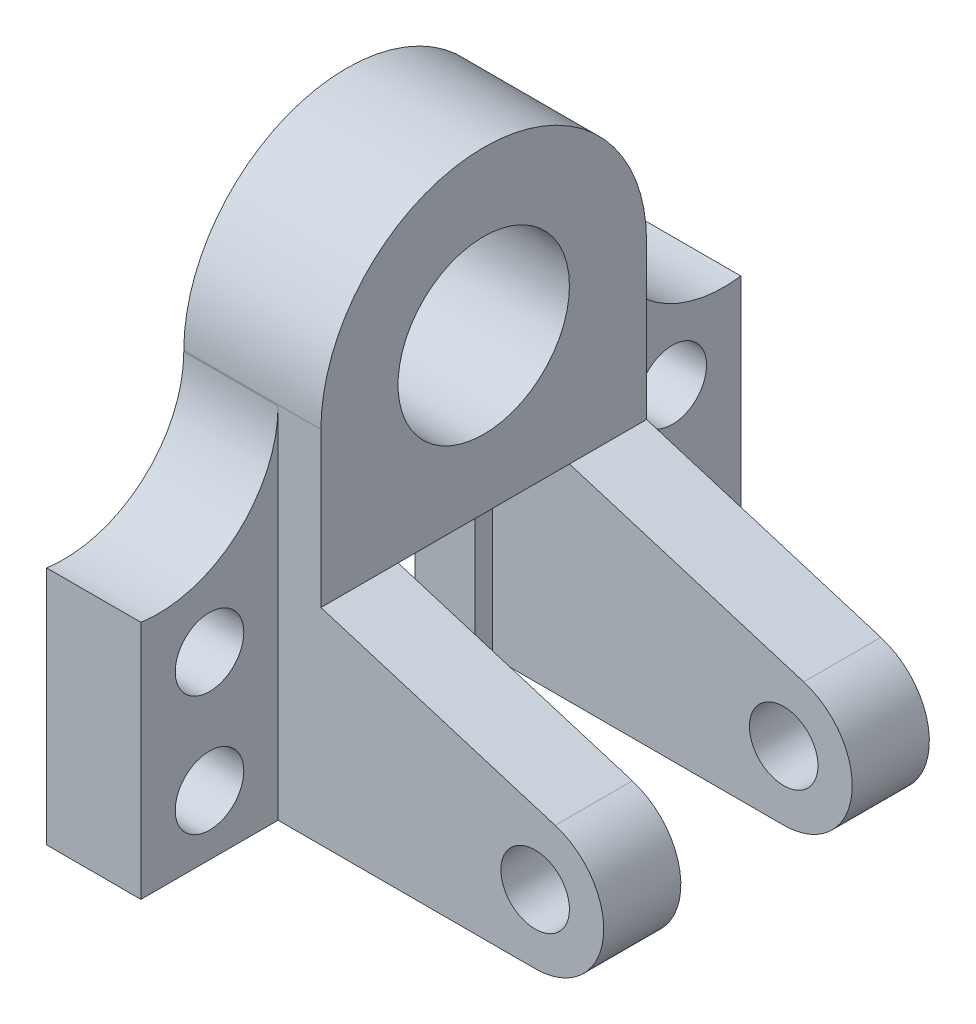
ISO-10303-21;
HEADER;
FILE_DESCRIPTION(('STEP AP214'),'2;1');
FILE_NAME('part.step','',(''),(''),'','','');
FILE_SCHEMA(('AUTOMOTIVE_DESIGN { 1 0 10303 214 1 1 1 1 }'));
ENDSEC;
DATA;
#1=APPLICATION_CONTEXT('core data for automotive mechanical design processes');
#2=APPLICATION_PROTOCOL_DEFINITION('international standard','automotive_design',2000,#1);
#3=PRODUCT_CONTEXT('',#1,'mechanical');
#4=PRODUCT('Part','Part','',(#3));
#5=PRODUCT_RELATED_PRODUCT_CATEGORY('part','',(#4));
#6=PRODUCT_DEFINITION_FORMATION('','',#4);
#7=PRODUCT_DEFINITION_CONTEXT('part definition',#1,'design');
#8=PRODUCT_DEFINITION('design','',#6,#7);
#9=PRODUCT_DEFINITION_SHAPE('','',#8);
#10=(LENGTH_UNIT() NAMED_UNIT(*) SI_UNIT(.MILLI.,.METRE.));
#11=(NAMED_UNIT(*) PLANE_ANGLE_UNIT() SI_UNIT($,.RADIAN.));
#12=(NAMED_UNIT(*) SI_UNIT($,.STERADIAN.) SOLID_ANGLE_UNIT());
#13=UNCERTAINTY_MEASURE_WITH_UNIT(LENGTH_MEASURE(1.E-05),#10,'distance_accuracy_value','');
#14=(GEOMETRIC_REPRESENTATION_CONTEXT(3) GLOBAL_UNCERTAINTY_ASSIGNED_CONTEXT((#13)) GLOBAL_UNIT_ASSIGNED_CONTEXT((#10,
#11,#12)) REPRESENTATION_CONTEXT('',''));
#15=CARTESIAN_POINT('',(0.,0.,0.));
#16=DIRECTION('',(0.,0.,1.));
#17=DIRECTION('',(1.,0.,0.));
#18=AXIS2_PLACEMENT_3D('',#15,#16,#17);
#19=CARTESIAN_POINT('',(32.,-36.,38.));
#20=DIRECTION('',(0.,1.,0.));
#21=DIRECTION('',(0.,0.,1.));
#22=AXIS2_PLACEMENT_3D('',#19,#20,#21);
#23=PLANE('',#22);
#24=DIRECTION('',(0.,0.,-1.));
#25=VECTOR('',#24,1.);
#26=CARTESIAN_POINT('',(14.,-36.,20.));
#27=LINE('',#26,#25);
#28=CARTESIAN_POINT('',(14.,-36.,20.));
#29=VERTEX_POINT('',#28);
#30=CARTESIAN_POINT('',(14.,-36.,16.));
#31=VERTEX_POINT('',#30);
#32=EDGE_CURVE('E181',#29,#31,#27,.T.);
#33=ORIENTED_EDGE('',*,*,#32,.T.);
#34=DIRECTION('',(-1.,0.,0.));
#35=VECTOR('',#34,1.);
#36=CARTESIAN_POINT('',(14.,-36.,16.));
#37=LINE('',#36,#35);
#38=CARTESIAN_POINT('',(0.,-36.,16.));
#39=VERTEX_POINT('',#38);
#40=EDGE_CURVE('E730',#31,#39,#37,.T.);
#41=ORIENTED_EDGE('',*,*,#40,.T.);
#42=DIRECTION('',(0.,0.,-1.));
#43=VECTOR('',#42,1.);
#44=CARTESIAN_POINT('',(0.,-36.,38.));
#45=LINE('',#44,#43);
#46=CARTESIAN_POINT('',(0.,-36.,-16.));
#47=VERTEX_POINT('',#46);
#48=EDGE_CURVE('E61',#39,#47,#45,.T.);
#49=ORIENTED_EDGE('',*,*,#48,.T.);
#50=DIRECTION('',(-1.,0.,0.));
#51=VECTOR('',#50,1.);
#52=CARTESIAN_POINT('',(14.,-36.,-16.));
#53=LINE('',#52,#51);
#54=CARTESIAN_POINT('',(14.,-36.,-16.));
#55=VERTEX_POINT('',#54);
#56=EDGE_CURVE('E57',#55,#47,#53,.T.);
#57=ORIENTED_EDGE('',*,*,#56,.F.);
#58=DIRECTION('',(0.,0.,-1.));
#59=VECTOR('',#58,1.);
#60=CARTESIAN_POINT('',(14.,-36.,-20.));
#61=LINE('',#60,#59);
#62=CARTESIAN_POINT('',(14.,-36.,-20.));
#63=VERTEX_POINT('',#62);
#64=EDGE_CURVE('E744',#55,#63,#61,.T.);
#65=ORIENTED_EDGE('',*,*,#64,.T.);
#66=DIRECTION('',(-1.,0.,0.));
#67=VECTOR('',#66,1.);
#68=CARTESIAN_POINT('',(32.,-36.,-20.));
#69=LINE('',#68,#67);
#70=CARTESIAN_POINT('',(32.,-36.,-20.));
#71=VERTEX_POINT('',#70);
#72=EDGE_CURVE('E368',#71,#63,#69,.T.);
#73=ORIENTED_EDGE('',*,*,#72,.F.);
#74=DIRECTION('',(0.,0.,-1.));
#75=VECTOR('',#74,1.);
#76=CARTESIAN_POINT('',(32.,-36.,38.));
#77=LINE('',#76,#75);
#78=CARTESIAN_POINT('',(32.,-36.,20.));
#79=VERTEX_POINT('',#78);
#80=EDGE_CURVE('E206',#79,#71,#77,.T.);
#81=ORIENTED_EDGE('',*,*,#80,.F.);
#82=DIRECTION('',(-1.,0.,0.));
#83=VECTOR('',#82,1.);
#84=CARTESIAN_POINT('',(32.,-36.,20.));
#85=LINE('',#84,#83);
#86=EDGE_CURVE('E200',#79,#29,#85,.T.);
#87=ORIENTED_EDGE('',*,*,#86,.T.);
#88=EDGE_LOOP('',(#33,#41,#49,#57,#65,#73,#81,#87));
#89=FACE_BOUND('',#88,.T.);
#90=ADVANCED_FACE('F41',(#89),#23,.F.);
#91=CARTESIAN_POINT('',(32.,0.,-38.));
#92=DIRECTION('',(0.,0.,1.));
#93=DIRECTION('',(0.,-1.,0.));
#94=AXIS2_PLACEMENT_3D('',#91,#92,#93);
#95=PLANE('',#94);
#96=DIRECTION('',(0.,-1.,0.));
#97=VECTOR('',#96,1.);
#98=CARTESIAN_POINT('',(22.,-0.28718707889796,-38.));
#99=LINE('',#98,#97);
#100=CARTESIAN_POINT('',(22.,-0.28718707889796,-38.));
#101=VERTEX_POINT('',#100);
#102=CARTESIAN_POINT('',(22.,-84.,-38.));
#103=VERTEX_POINT('',#102);
#104=EDGE_CURVE('E238',#101,#103,#99,.T.);
#105=ORIENTED_EDGE('',*,*,#104,.F.);
#106=DIRECTION('',(-1.,0.,0.));
#107=VECTOR('',#106,1.);
#108=CARTESIAN_POINT('',(22.,-0.28718707889796,-38.));
#109=LINE('',#108,#107);
#110=CARTESIAN_POINT('',(0.,-0.287187078897948,-38.));
#111=VERTEX_POINT('',#110);
#112=EDGE_CURVE('E260',#101,#111,#109,.T.);
#113=ORIENTED_EDGE('',*,*,#112,.T.);
#114=DIRECTION('',(0.,1.,0.));
#115=VECTOR('',#114,1.);
#116=CARTESIAN_POINT('',(0.,0.,-38.));
#117=LINE('',#116,#115);
#118=CARTESIAN_POINT('',(0.,0.,-38.));
#119=VERTEX_POINT('',#118);
#120=EDGE_CURVE('E307',#111,#119,#117,.T.);
#121=ORIENTED_EDGE('',*,*,#120,.T.);
#122=DIRECTION('',(-1.,0.,0.));
#123=VECTOR('',#122,1.);
#124=CARTESIAN_POINT('',(32.,0.,-38.));
#125=LINE('',#124,#123);
#126=CARTESIAN_POINT('',(32.,0.,-38.));
#127=VERTEX_POINT('',#126);
#128=EDGE_CURVE('E47',#127,#119,#125,.T.);
#129=ORIENTED_EDGE('',*,*,#128,.F.);
#130=DIRECTION('',(0.,1.,0.));
#131=VECTOR('',#130,1.);
#132=CARTESIAN_POINT('',(32.,0.,-38.));
#133=LINE('',#132,#131);
#134=CARTESIAN_POINT('',(32.,-36.,-38.));
#135=VERTEX_POINT('',#134);
#136=EDGE_CURVE('E313',#135,#127,#133,.T.);
#137=ORIENTED_EDGE('',*,*,#136,.F.);
#138=DIRECTION('',(-0.956390801813646,0.292090113160734,0.));
#139=VECTOR('',#138,1.);
#140=CARTESIAN_POINT('',(86.6734418105717,-52.6977471709817,-38.));
#141=LINE('',#140,#139);
#142=CARTESIAN_POINT('',(86.6734418105717,-52.6977471709817,-38.));
#143=VERTEX_POINT('',#142);
#144=EDGE_CURVE('E348',#143,#135,#141,.T.);
#145=ORIENTED_EDGE('',*,*,#144,.F.);
#146=CARTESIAN_POINT('',(82.,-68.,-38.));
#147=DIRECTION('',(0.,0.,1.));
#148=DIRECTION('',(1.,0.,0.));
#149=AXIS2_PLACEMENT_3D('',#146,#147,#148);
#150=CIRCLE('',#149,16.);
#151=CARTESIAN_POINT('',(82.,-84.,-38.));
#152=VERTEX_POINT('',#151);
#153=EDGE_CURVE('E352',#152,#143,#150,.T.);
#154=ORIENTED_EDGE('',*,*,#153,.F.);
#155=DIRECTION('',(1.,0.,0.));
#156=VECTOR('',#155,1.);
#157=CARTESIAN_POINT('',(0.,-84.,-38.));
#158=LINE('',#157,#156);
#159=EDGE_CURVE('E365',#103,#152,#158,.T.);
#160=ORIENTED_EDGE('',*,*,#159,.F.);
#161=EDGE_LOOP('',(#105,#113,#121,#129,#137,#145,#154,#160));
#162=FACE_BOUND('',#161,.T.);
#163=CARTESIAN_POINT('',(82.,-68.,-38.));
#164=DIRECTION('',(0.,0.,1.));
#165=DIRECTION('',(1.,0.,0.));
#166=AXIS2_PLACEMENT_3D('',#163,#164,#165);
#167=CIRCLE('',#166,8.00000000000001);
#168=CARTESIAN_POINT('',(90.,-68.,-38.));
#169=VERTEX_POINT('',#168);
#170=EDGE_CURVE('E373',#169,#169,#167,.T.);
#171=ORIENTED_EDGE('',*,*,#170,.T.);
#172=EDGE_LOOP('',(#171));
#173=FACE_BOUND('',#172,.T.);
#174=ADVANCED_FACE('F350',(#162,#173),#95,.F.);
#175=CARTESIAN_POINT('',(32.,0.,0.));
#176=DIRECTION('',(1.,0.,0.));
#177=DIRECTION('',(0.,0.,-1.));
#178=AXIS2_PLACEMENT_3D('',#175,#176,#177);
#179=PLANE('',#178);
#180=CARTESIAN_POINT('',(32.,0.,0.));
#181=DIRECTION('',(1.,0.,0.));
#182=DIRECTION('',(0.,0.,-1.));
#183=AXIS2_PLACEMENT_3D('',#180,#181,#182);
#184=CIRCLE('',#183,38.);
#185=CARTESIAN_POINT('',(32.,0.,38.));
#186=VERTEX_POINT('',#185);
#187=EDGE_CURVE('E301',#127,#186,#184,.T.);
#188=ORIENTED_EDGE('',*,*,#187,.T.);
#189=DIRECTION('',(0.,-1.,0.));
#190=VECTOR('',#189,1.);
#191=CARTESIAN_POINT('',(32.,0.,38.));
#192=LINE('',#191,#190);
#193=CARTESIAN_POINT('',(32.,-36.,38.));
#194=VERTEX_POINT('',#193);
#195=EDGE_CURVE('E308',#186,#194,#192,.T.);
#196=ORIENTED_EDGE('',*,*,#195,.T.);
#197=EDGE_CURVE('E310',#194,#79,#77,.T.);
#198=ORIENTED_EDGE('',*,*,#197,.T.);
#199=ORIENTED_EDGE('',*,*,#80,.T.);
#200=DIRECTION('',(0.,0.,1.));
#201=VECTOR('',#200,1.);
#202=CARTESIAN_POINT('',(32.,-36.,-38.));
#203=LINE('',#202,#201);
#204=EDGE_CURVE('E342',#135,#71,#203,.T.);
#205=ORIENTED_EDGE('',*,*,#204,.F.);
#206=ORIENTED_EDGE('',*,*,#136,.T.);
#207=EDGE_LOOP('',(#188,#196,#198,#199,#205,#206));
#208=FACE_BOUND('',#207,.T.);
#209=CARTESIAN_POINT('',(32.,0.,0.));
#210=DIRECTION('',(1.,0.,0.));
#211=DIRECTION('',(0.,0.,-1.));
#212=AXIS2_PLACEMENT_3D('',#209,#210,#211);
#213=CIRCLE('',#212,20.);
#214=CARTESIAN_POINT('',(32.,0.,-20.));
#215=VERTEX_POINT('',#214);
#216=EDGE_CURVE('E300',#215,#215,#213,.T.);
#217=ORIENTED_EDGE('',*,*,#216,.F.);
#218=EDGE_LOOP('',(#217));
#219=FACE_BOUND('',#218,.T.);
#220=ADVANCED_FACE('F343',(#208,#219),#179,.T.);
#221=CARTESIAN_POINT('',(0.,0.,0.));
#222=DIRECTION('',(1.,0.,0.));
#223=DIRECTION('',(0.,0.,-1.));
#224=AXIS2_PLACEMENT_3D('',#221,#222,#223);
#225=PLANE('',#224);
#226=ORIENTED_EDGE('',*,*,#48,.F.);
#227=DIRECTION('',(0.,-1.,0.));
#228=VECTOR('',#227,1.);
#229=CARTESIAN_POINT('',(0.,-36.,16.));
#230=LINE('',#229,#228);
#231=CARTESIAN_POINT('',(0.,-84.,16.));
#232=VERTEX_POINT('',#231);
#233=EDGE_CURVE('E205',#39,#232,#230,.T.);
#234=ORIENTED_EDGE('',*,*,#233,.T.);
#235=DIRECTION('',(0.,0.,-1.));
#236=VECTOR('',#235,1.);
#237=CARTESIAN_POINT('',(0.,-84.,38.));
#238=LINE('',#237,#236);
#239=CARTESIAN_POINT('',(0.,-84.,70.));
#240=VERTEX_POINT('',#239);
#241=EDGE_CURVE('E280',#240,#232,#238,.T.);
#242=ORIENTED_EDGE('',*,*,#241,.F.);
#243=DIRECTION('',(0.,-1.,0.));
#244=VECTOR('',#243,1.);
#245=CARTESIAN_POINT('',(0.,-28.,70.));
#246=LINE('',#245,#244);
#247=CARTESIAN_POINT('',(0.,-28.,70.));
#248=VERTEX_POINT('',#247);
#249=EDGE_CURVE('E288',#248,#240,#246,.T.);
#250=ORIENTED_EDGE('',*,*,#249,.F.);
#251=CARTESIAN_POINT('',(0.,-0.287187078897969,66.));
#252=DIRECTION('',(-1.,0.,0.));
#253=DIRECTION('',(0.,0.,-1.));
#254=AXIS2_PLACEMENT_3D('',#251,#252,#253);
#255=CIRCLE('',#254,28.);
#256=CARTESIAN_POINT('',(0.,-0.287187078897969,38.));
#257=VERTEX_POINT('',#256);
#258=EDGE_CURVE('E269',#257,#248,#255,.T.);
#259=ORIENTED_EDGE('',*,*,#258,.F.);
#260=DIRECTION('',(0.,-1.,0.));
#261=VECTOR('',#260,1.);
#262=CARTESIAN_POINT('',(0.,0.,38.));
#263=LINE('',#262,#261);
#264=CARTESIAN_POINT('',(0.,0.,38.));
#265=VERTEX_POINT('',#264);
#266=EDGE_CURVE('E312',#265,#257,#263,.T.);
#267=ORIENTED_EDGE('',*,*,#266,.F.);
#268=CARTESIAN_POINT('',(0.,0.,0.));
#269=DIRECTION('',(1.,0.,0.));
#270=DIRECTION('',(0.,0.,-1.));
#271=AXIS2_PLACEMENT_3D('',#268,#269,#270);
#272=CIRCLE('',#271,38.);
#273=EDGE_CURVE('E299',#119,#265,#272,.T.);
#274=ORIENTED_EDGE('',*,*,#273,.F.);
#275=ORIENTED_EDGE('',*,*,#120,.F.);
#276=CARTESIAN_POINT('',(0.,-0.287187078897953,-66.));
#277=DIRECTION('',(-1.,0.,0.));
#278=DIRECTION('',(0.,0.,1.));
#279=AXIS2_PLACEMENT_3D('',#276,#277,#278);
#280=CIRCLE('',#279,28.);
#281=CARTESIAN_POINT('',(0.,-28.,-70.));
#282=VERTEX_POINT('',#281);
#283=EDGE_CURVE('E234',#282,#111,#280,.T.);
#284=ORIENTED_EDGE('',*,*,#283,.F.);
#285=DIRECTION('',(0.,1.,0.));
#286=VECTOR('',#285,1.);
#287=CARTESIAN_POINT('',(0.,-28.,-70.));
#288=LINE('',#287,#286);
#289=CARTESIAN_POINT('',(0.,-84.,-70.));
#290=VERTEX_POINT('',#289);
#291=EDGE_CURVE('E241',#290,#282,#288,.T.);
#292=ORIENTED_EDGE('',*,*,#291,.F.);
#293=DIRECTION('',(0.,0.,-1.));
#294=VECTOR('',#293,1.);
#295=CARTESIAN_POINT('',(0.,-84.,-38.));
#296=LINE('',#295,#294);
#297=CARTESIAN_POINT('',(0.,-84.,-16.));
#298=VERTEX_POINT('',#297);
#299=EDGE_CURVE('E247',#298,#290,#296,.T.);
#300=ORIENTED_EDGE('',*,*,#299,.F.);
#301=DIRECTION('',(0.,1.,0.));
#302=VECTOR('',#301,1.);
#303=CARTESIAN_POINT('',(0.,-84.,-16.));
#304=LINE('',#303,#302);
#305=EDGE_CURVE('E733',#298,#47,#304,.T.);
#306=ORIENTED_EDGE('',*,*,#305,.T.);
#307=EDGE_LOOP('',(#226,#234,#242,#250,#259,#267,#274,#275,#284,#292,#300,#306));
#308=FACE_BOUND('',#307,.T.);
#309=CARTESIAN_POINT('',(0.,0.,0.));
#310=DIRECTION('',(1.,0.,0.));
#311=DIRECTION('',(0.,0.,-1.));
#312=AXIS2_PLACEMENT_3D('',#309,#310,#311);
#313=CIRCLE('',#312,20.);
#314=CARTESIAN_POINT('',(0.,0.,-20.));
#315=VERTEX_POINT('',#314);
#316=EDGE_CURVE('E296',#315,#315,#313,.T.);
#317=ORIENTED_EDGE('',*,*,#316,.T.);
#318=EDGE_LOOP('',(#317));
#319=FACE_BOUND('',#318,.T.);
#320=CARTESIAN_POINT('',(0.,-42.,54.));
#321=DIRECTION('',(1.,0.,0.));
#322=DIRECTION('',(0.,0.,-1.));
#323=AXIS2_PLACEMENT_3D('',#320,#321,#322);
#324=CIRCLE('',#323,8.);
#325=CARTESIAN_POINT('',(0.,-42.,46.));
#326=VERTEX_POINT('',#325);
#327=EDGE_CURVE('E262',#326,#326,#324,.T.);
#328=ORIENTED_EDGE('',*,*,#327,.T.);
#329=EDGE_LOOP('',(#328));
#330=FACE_BOUND('',#329,.T.);
#331=CARTESIAN_POINT('',(0.,-70.,54.));
#332=DIRECTION('',(1.,0.,0.));
#333=DIRECTION('',(0.,0.,-1.));
#334=AXIS2_PLACEMENT_3D('',#331,#332,#333);
#335=CIRCLE('',#334,8.);
#336=CARTESIAN_POINT('',(0.,-70.,46.));
#337=VERTEX_POINT('',#336);
#338=EDGE_CURVE('E257',#337,#337,#335,.T.);
#339=ORIENTED_EDGE('',*,*,#338,.T.);
#340=EDGE_LOOP('',(#339));
#341=FACE_BOUND('',#340,.T.);
#342=CARTESIAN_POINT('',(0.,-70.,-54.));
#343=DIRECTION('',(1.,0.,0.));
#344=DIRECTION('',(0.,0.,1.));
#345=AXIS2_PLACEMENT_3D('',#342,#343,#344);
#346=CIRCLE('',#345,8.);
#347=CARTESIAN_POINT('',(0.,-70.,-46.));
#348=VERTEX_POINT('',#347);
#349=EDGE_CURVE('E228',#348,#348,#346,.T.);
#350=ORIENTED_EDGE('',*,*,#349,.T.);
#351=EDGE_LOOP('',(#350));
#352=FACE_BOUND('',#351,.T.);
#353=CARTESIAN_POINT('',(0.,-42.,-54.));
#354=DIRECTION('',(1.,0.,0.));
#355=DIRECTION('',(0.,0.,1.));
#356=AXIS2_PLACEMENT_3D('',#353,#354,#355);
#357=CIRCLE('',#356,8.);
#358=CARTESIAN_POINT('',(0.,-42.,-46.));
#359=VERTEX_POINT('',#358);
#360=EDGE_CURVE('E223',#359,#359,#357,.T.);
#361=ORIENTED_EDGE('',*,*,#360,.T.);
#362=EDGE_LOOP('',(#361));
#363=FACE_BOUND('',#362,.T.);
#364=ADVANCED_FACE('F328',(#308,#319,#330,#341,#352,#363),#225,.F.);
#365=CARTESIAN_POINT('',(32.,0.,0.));
#366=DIRECTION('',(-1.,0.,0.));
#367=DIRECTION('',(0.,0.,1.));
#368=AXIS2_PLACEMENT_3D('',#365,#366,#367);
#369=CYLINDRICAL_SURFACE('',#368,38.);
#370=ORIENTED_EDGE('',*,*,#273,.T.);
#371=DIRECTION('',(-1.,0.,0.));
#372=VECTOR('',#371,1.);
#373=CARTESIAN_POINT('',(32.,0.,38.));
#374=LINE('',#373,#372);
#375=EDGE_CURVE('E11',#186,#265,#374,.T.);
#376=ORIENTED_EDGE('',*,*,#375,.F.);
#377=ORIENTED_EDGE('',*,*,#187,.F.);
#378=ORIENTED_EDGE('',*,*,#128,.T.);
#379=EDGE_LOOP('',(#370,#376,#377,#378));
#380=FACE_BOUND('',#379,.T.);
#381=ADVANCED_FACE('F43',(#380),#369,.T.);
#382=CARTESIAN_POINT('',(32.,0.,38.));
#383=DIRECTION('',(0.,0.,-1.));
#384=DIRECTION('',(0.,1.,0.));
#385=AXIS2_PLACEMENT_3D('',#382,#383,#384);
#386=PLANE('',#385);
#387=DIRECTION('',(-1.,0.,0.));
#388=VECTOR('',#387,1.);
#389=CARTESIAN_POINT('',(22.,-0.287187078897969,38.));
#390=LINE('',#389,#388);
#391=CARTESIAN_POINT('',(22.,-0.287187078897969,38.));
#392=VERTEX_POINT('',#391);
#393=EDGE_CURVE('E282',#392,#257,#390,.T.);
#394=ORIENTED_EDGE('',*,*,#393,.F.);
#395=DIRECTION('',(0.,1.,0.));
#396=VECTOR('',#395,1.);
#397=CARTESIAN_POINT('',(22.,-0.287187078897969,38.));
#398=LINE('',#397,#396);
#399=CARTESIAN_POINT('',(22.,-84.,38.));
#400=VERTEX_POINT('',#399);
#401=EDGE_CURVE('E281',#400,#392,#398,.T.);
#402=ORIENTED_EDGE('',*,*,#401,.F.);
#403=DIRECTION('',(1.,0.,0.));
#404=VECTOR('',#403,1.);
#405=CARTESIAN_POINT('',(0.,-84.,38.));
#406=LINE('',#405,#404);
#407=CARTESIAN_POINT('',(82.,-84.,38.));
#408=VERTEX_POINT('',#407);
#409=EDGE_CURVE('E208',#400,#408,#406,.T.);
#410=ORIENTED_EDGE('',*,*,#409,.T.);
#411=CARTESIAN_POINT('',(82.,-68.,38.));
#412=DIRECTION('',(0.,0.,1.));
#413=DIRECTION('',(1.,0.,0.));
#414=AXIS2_PLACEMENT_3D('',#411,#412,#413);
#415=CIRCLE('',#414,16.);
#416=CARTESIAN_POINT('',(86.6734418105717,-52.6977471709817,38.));
#417=VERTEX_POINT('',#416);
#418=EDGE_CURVE('E211',#408,#417,#415,.T.);
#419=ORIENTED_EDGE('',*,*,#418,.T.);
#420=DIRECTION('',(-0.956390801813646,0.292090113160734,0.));
#421=VECTOR('',#420,1.);
#422=CARTESIAN_POINT('',(86.6734418105717,-52.6977471709817,38.));
#423=LINE('',#422,#421);
#424=EDGE_CURVE('E225',#417,#194,#423,.T.);
#425=ORIENTED_EDGE('',*,*,#424,.T.);
#426=ORIENTED_EDGE('',*,*,#195,.F.);
#427=ORIENTED_EDGE('',*,*,#375,.T.);
#428=ORIENTED_EDGE('',*,*,#266,.T.);
#429=EDGE_LOOP('',(#394,#402,#410,#419,#425,#426,#427,#428));
#430=FACE_BOUND('',#429,.T.);
#431=CARTESIAN_POINT('',(82.,-68.,38.));
#432=DIRECTION('',(0.,0.,1.));
#433=DIRECTION('',(1.,0.,0.));
#434=AXIS2_PLACEMENT_3D('',#431,#432,#433);
#435=CIRCLE('',#434,8.00000000000001);
#436=CARTESIAN_POINT('',(90.,-68.,38.));
#437=VERTEX_POINT('',#436);
#438=EDGE_CURVE('E384',#437,#437,#435,.T.);
#439=ORIENTED_EDGE('',*,*,#438,.F.);
#440=EDGE_LOOP('',(#439));
#441=FACE_BOUND('',#440,.T.);
#442=ADVANCED_FACE('F333',(#430,#441),#386,.F.);
#443=CARTESIAN_POINT('',(32.,0.,0.));
#444=DIRECTION('',(-1.,0.,0.));
#445=DIRECTION('',(0.,0.,1.));
#446=AXIS2_PLACEMENT_3D('',#443,#444,#445);
#447=CYLINDRICAL_SURFACE('',#446,20.);
#448=ORIENTED_EDGE('',*,*,#216,.T.);
#449=EDGE_LOOP('',(#448));
#450=FACE_BOUND('',#449,.T.);
#451=ORIENTED_EDGE('',*,*,#316,.F.);
#452=EDGE_LOOP('',(#451));
#453=FACE_BOUND('',#452,.T.);
#454=ADVANCED_FACE('F423',(#450,#453),#447,.F.);
#455=CARTESIAN_POINT('',(22.,-0.287187078897969,66.));
#456=DIRECTION('',(1.,0.,0.));
#457=DIRECTION('',(0.,0.,-1.));
#458=AXIS2_PLACEMENT_3D('',#455,#456,#457);
#459=PLANE('',#458);
#460=CARTESIAN_POINT('',(22.,-42.,54.));
#461=DIRECTION('',(1.,0.,0.));
#462=DIRECTION('',(0.,0.,-1.));
#463=AXIS2_PLACEMENT_3D('',#460,#461,#462);
#464=CIRCLE('',#463,8.);
#465=CARTESIAN_POINT('',(22.,-42.,46.));
#466=VERTEX_POINT('',#465);
#467=EDGE_CURVE('E270',#466,#466,#464,.T.);
#468=ORIENTED_EDGE('',*,*,#467,.F.);
#469=EDGE_LOOP('',(#468));
#470=FACE_BOUND('',#469,.T.);
#471=CARTESIAN_POINT('',(22.,-0.287187078897969,66.));
#472=DIRECTION('',(-1.,0.,0.));
#473=DIRECTION('',(0.,0.,-1.));
#474=AXIS2_PLACEMENT_3D('',#471,#472,#473);
#475=CIRCLE('',#474,28.);
#476=CARTESIAN_POINT('',(22.,-28.,70.));
#477=VERTEX_POINT('',#476);
#478=EDGE_CURVE('E272',#392,#477,#475,.T.);
#479=ORIENTED_EDGE('',*,*,#478,.T.);
#480=DIRECTION('',(0.,-1.,0.));
#481=VECTOR('',#480,1.);
#482=CARTESIAN_POINT('',(22.,-28.,70.));
#483=LINE('',#482,#481);
#484=CARTESIAN_POINT('',(22.,-84.,70.));
#485=VERTEX_POINT('',#484);
#486=EDGE_CURVE('E277',#477,#485,#483,.T.);
#487=ORIENTED_EDGE('',*,*,#486,.T.);
#488=DIRECTION('',(0.,0.,-1.));
#489=VECTOR('',#488,1.);
#490=CARTESIAN_POINT('',(22.,-84.,38.));
#491=LINE('',#490,#489);
#492=EDGE_CURVE('E276',#485,#400,#491,.T.);
#493=ORIENTED_EDGE('',*,*,#492,.T.);
#494=ORIENTED_EDGE('',*,*,#401,.T.);
#495=EDGE_LOOP('',(#479,#487,#493,#494));
#496=FACE_BOUND('',#495,.T.);
#497=CARTESIAN_POINT('',(22.,-70.,54.));
#498=DIRECTION('',(1.,0.,0.));
#499=DIRECTION('',(0.,0.,-1.));
#500=AXIS2_PLACEMENT_3D('',#497,#498,#499);
#501=CIRCLE('',#500,8.);
#502=CARTESIAN_POINT('',(22.,-70.,46.));
#503=VERTEX_POINT('',#502);
#504=EDGE_CURVE('E261',#503,#503,#501,.T.);
#505=ORIENTED_EDGE('',*,*,#504,.F.);
#506=EDGE_LOOP('',(#505));
#507=FACE_BOUND('',#506,.T.);
#508=ADVANCED_FACE('F430',(#470,#496,#507),#459,.T.);
#509=CARTESIAN_POINT('',(22.,-0.287187078897969,66.));
#510=DIRECTION('',(-1.,0.,0.));
#511=DIRECTION('',(0.,0.,1.));
#512=AXIS2_PLACEMENT_3D('',#509,#510,#511);
#513=CYLINDRICAL_SURFACE('',#512,28.);
#514=ORIENTED_EDGE('',*,*,#258,.T.);
#515=DIRECTION('',(-1.,0.,0.));
#516=VECTOR('',#515,1.);
#517=CARTESIAN_POINT('',(22.,-28.,70.));
#518=LINE('',#517,#516);
#519=EDGE_CURVE('E291',#477,#248,#518,.T.);
#520=ORIENTED_EDGE('',*,*,#519,.F.);
#521=ORIENTED_EDGE('',*,*,#478,.F.);
#522=ORIENTED_EDGE('',*,*,#393,.T.);
#523=EDGE_LOOP('',(#514,#520,#521,#522));
#524=FACE_BOUND('',#523,.T.);
#525=ADVANCED_FACE('F438',(#524),#513,.F.);
#526=CARTESIAN_POINT('',(22.,-28.,70.));
#527=DIRECTION('',(0.,0.,-1.));
#528=DIRECTION('',(0.,1.,0.));
#529=AXIS2_PLACEMENT_3D('',#526,#527,#528);
#530=PLANE('',#529);
#531=ORIENTED_EDGE('',*,*,#249,.T.);
#532=DIRECTION('',(-1.,0.,0.));
#533=VECTOR('',#532,1.);
#534=CARTESIAN_POINT('',(22.,-84.,70.));
#535=LINE('',#534,#533);
#536=EDGE_CURVE('E289',#485,#240,#535,.T.);
#537=ORIENTED_EDGE('',*,*,#536,.F.);
#538=ORIENTED_EDGE('',*,*,#486,.F.);
#539=ORIENTED_EDGE('',*,*,#519,.T.);
#540=EDGE_LOOP('',(#531,#537,#538,#539));
#541=FACE_BOUND('',#540,.T.);
#542=ADVANCED_FACE('F445',(#541),#530,.F.);
#543=CARTESIAN_POINT('',(22.,-84.,38.));
#544=DIRECTION('',(0.,1.,0.));
#545=DIRECTION('',(0.,0.,1.));
#546=AXIS2_PLACEMENT_3D('',#543,#544,#545);
#547=PLANE('',#546);
#548=ORIENTED_EDGE('',*,*,#241,.T.);
#549=DIRECTION('',(-1.,0.,0.));
#550=VECTOR('',#549,1.);
#551=CARTESIAN_POINT('',(14.,-84.,16.));
#552=LINE('',#551,#550);
#553=CARTESIAN_POINT('',(14.,-84.,16.));
#554=VERTEX_POINT('',#553);
#555=EDGE_CURVE('E726',#554,#232,#552,.T.);
#556=ORIENTED_EDGE('',*,*,#555,.F.);
#557=DIRECTION('',(0.,0.,1.));
#558=VECTOR('',#557,1.);
#559=CARTESIAN_POINT('',(14.,-84.,20.));
#560=LINE('',#559,#558);
#561=CARTESIAN_POINT('',(14.,-84.,20.));
#562=VERTEX_POINT('',#561);
#563=EDGE_CURVE('E732',#554,#562,#560,.T.);
#564=ORIENTED_EDGE('',*,*,#563,.T.);
#565=DIRECTION('',(1.,0.,0.));
#566=VECTOR('',#565,1.);
#567=CARTESIAN_POINT('',(0.,-84.,20.));
#568=LINE('',#567,#566);
#569=CARTESIAN_POINT('',(82.,-84.,20.));
#570=VERTEX_POINT('',#569);
#571=EDGE_CURVE('E203',#562,#570,#568,.T.);
#572=ORIENTED_EDGE('',*,*,#571,.T.);
#573=DIRECTION('',(0.,0.,-1.));
#574=VECTOR('',#573,1.);
#575=CARTESIAN_POINT('',(82.,-84.,38.));
#576=LINE('',#575,#574);
#577=EDGE_CURVE('E222',#408,#570,#576,.T.);
#578=ORIENTED_EDGE('',*,*,#577,.F.);
#579=ORIENTED_EDGE('',*,*,#409,.F.);
#580=ORIENTED_EDGE('',*,*,#492,.F.);
#581=ORIENTED_EDGE('',*,*,#536,.T.);
#582=EDGE_LOOP('',(#548,#556,#564,#572,#578,#579,#580,#581));
#583=FACE_BOUND('',#582,.T.);
#584=ADVANCED_FACE('F446',(#583),#547,.F.);
#585=CARTESIAN_POINT('',(22.,-42.,54.));
#586=DIRECTION('',(-1.,0.,0.));
#587=DIRECTION('',(0.,0.,1.));
#588=AXIS2_PLACEMENT_3D('',#585,#586,#587);
#589=CYLINDRICAL_SURFACE('',#588,8.);
#590=ORIENTED_EDGE('',*,*,#467,.T.);
#591=EDGE_LOOP('',(#590));
#592=FACE_BOUND('',#591,.T.);
#593=ORIENTED_EDGE('',*,*,#327,.F.);
#594=EDGE_LOOP('',(#593));
#595=FACE_BOUND('',#594,.T.);
#596=ADVANCED_FACE('F448',(#592,#595),#589,.F.);
#597=CARTESIAN_POINT('',(22.,-70.,54.));
#598=DIRECTION('',(-1.,0.,0.));
#599=DIRECTION('',(0.,0.,1.));
#600=AXIS2_PLACEMENT_3D('',#597,#598,#599);
#601=CYLINDRICAL_SURFACE('',#600,8.);
#602=ORIENTED_EDGE('',*,*,#504,.T.);
#603=EDGE_LOOP('',(#602));
#604=FACE_BOUND('',#603,.T.);
#605=ORIENTED_EDGE('',*,*,#338,.F.);
#606=EDGE_LOOP('',(#605));
#607=FACE_BOUND('',#606,.T.);
#608=ADVANCED_FACE('F454',(#604,#607),#601,.F.);
#609=CARTESIAN_POINT('',(22.,-0.287187078897953,-66.));
#610=DIRECTION('',(-1.,0.,0.));
#611=DIRECTION('',(0.,0.,1.));
#612=AXIS2_PLACEMENT_3D('',#609,#610,#611);
#613=PLANE('',#612);
#614=CARTESIAN_POINT('',(22.,-0.287187078897953,-66.));
#615=DIRECTION('',(-1.,0.,0.));
#616=DIRECTION('',(0.,0.,1.));
#617=AXIS2_PLACEMENT_3D('',#614,#615,#616);
#618=CIRCLE('',#617,28.);
#619=CARTESIAN_POINT('',(22.,-28.,-70.));
#620=VERTEX_POINT('',#619);
#621=EDGE_CURVE('E236',#620,#101,#618,.T.);
#622=ORIENTED_EDGE('',*,*,#621,.T.);
#623=ORIENTED_EDGE('',*,*,#104,.T.);
#624=DIRECTION('',(0.,0.,-1.));
#625=VECTOR('',#624,1.);
#626=CARTESIAN_POINT('',(22.,-84.,-38.));
#627=LINE('',#626,#625);
#628=CARTESIAN_POINT('',(22.,-84.,-70.));
#629=VERTEX_POINT('',#628);
#630=EDGE_CURVE('E242',#103,#629,#627,.T.);
#631=ORIENTED_EDGE('',*,*,#630,.T.);
#632=DIRECTION('',(0.,1.,0.));
#633=VECTOR('',#632,1.);
#634=CARTESIAN_POINT('',(22.,-28.,-70.));
#635=LINE('',#634,#633);
#636=EDGE_CURVE('E244',#629,#620,#635,.T.);
#637=ORIENTED_EDGE('',*,*,#636,.T.);
#638=EDGE_LOOP('',(#622,#623,#631,#637));
#639=FACE_BOUND('',#638,.T.);
#640=CARTESIAN_POINT('',(22.,-70.,-54.));
#641=DIRECTION('',(1.,0.,0.));
#642=DIRECTION('',(0.,0.,1.));
#643=AXIS2_PLACEMENT_3D('',#640,#641,#642);
#644=CIRCLE('',#643,8.);
#645=CARTESIAN_POINT('',(22.,-70.,-46.));
#646=VERTEX_POINT('',#645);
#647=EDGE_CURVE('E235',#646,#646,#644,.T.);
#648=ORIENTED_EDGE('',*,*,#647,.F.);
#649=EDGE_LOOP('',(#648));
#650=FACE_BOUND('',#649,.T.);
#651=CARTESIAN_POINT('',(22.,-42.,-54.));
#652=DIRECTION('',(1.,0.,0.));
#653=DIRECTION('',(0.,0.,1.));
#654=AXIS2_PLACEMENT_3D('',#651,#652,#653);
#655=CIRCLE('',#654,8.);
#656=CARTESIAN_POINT('',(22.,-42.,-46.));
#657=VERTEX_POINT('',#656);
#658=EDGE_CURVE('E226',#657,#657,#655,.T.);
#659=ORIENTED_EDGE('',*,*,#658,.F.);
#660=EDGE_LOOP('',(#659));
#661=FACE_BOUND('',#660,.T.);
#662=ADVANCED_FACE('F459',(#639,#650,#661),#613,.F.);
#663=CARTESIAN_POINT('',(22.,-0.287187078897953,-66.));
#664=DIRECTION('',(-1.,0.,0.));
#665=DIRECTION('',(0.,0.,1.));
#666=AXIS2_PLACEMENT_3D('',#663,#664,#665);
#667=CYLINDRICAL_SURFACE('',#666,28.);
#668=ORIENTED_EDGE('',*,*,#283,.T.);
#669=ORIENTED_EDGE('',*,*,#112,.F.);
#670=ORIENTED_EDGE('',*,*,#621,.F.);
#671=DIRECTION('',(-1.,0.,0.));
#672=VECTOR('',#671,1.);
#673=CARTESIAN_POINT('',(22.,-28.,-70.));
#674=LINE('',#673,#672);
#675=EDGE_CURVE('E250',#620,#282,#674,.T.);
#676=ORIENTED_EDGE('',*,*,#675,.T.);
#677=EDGE_LOOP('',(#668,#669,#670,#676));
#678=FACE_BOUND('',#677,.T.);
#679=ADVANCED_FACE('F461',(#678),#667,.F.);
#680=CARTESIAN_POINT('',(22.,-84.,-38.));
#681=DIRECTION('',(0.,1.,0.));
#682=DIRECTION('',(0.,0.,1.));
#683=AXIS2_PLACEMENT_3D('',#680,#681,#682);
#684=PLANE('',#683);
#685=ORIENTED_EDGE('',*,*,#299,.T.);
#686=DIRECTION('',(-1.,0.,0.));
#687=VECTOR('',#686,1.);
#688=CARTESIAN_POINT('',(22.,-84.,-70.));
#689=LINE('',#688,#687);
#690=EDGE_CURVE('E255',#629,#290,#689,.T.);
#691=ORIENTED_EDGE('',*,*,#690,.F.);
#692=ORIENTED_EDGE('',*,*,#630,.F.);
#693=ORIENTED_EDGE('',*,*,#159,.T.);
#694=DIRECTION('',(0.,0.,1.));
#695=VECTOR('',#694,1.);
#696=CARTESIAN_POINT('',(82.,-84.,-38.));
#697=LINE('',#696,#695);
#698=CARTESIAN_POINT('',(82.,-84.,-20.));
#699=VERTEX_POINT('',#698);
#700=EDGE_CURVE('E354',#152,#699,#697,.T.);
#701=ORIENTED_EDGE('',*,*,#700,.T.);
#702=DIRECTION('',(1.,0.,0.));
#703=VECTOR('',#702,1.);
#704=CARTESIAN_POINT('',(0.,-84.,-20.));
#705=LINE('',#704,#703);
#706=CARTESIAN_POINT('',(14.,-84.,-20.));
#707=VERTEX_POINT('',#706);
#708=EDGE_CURVE('E367',#707,#699,#705,.T.);
#709=ORIENTED_EDGE('',*,*,#708,.F.);
#710=DIRECTION('',(0.,0.,1.));
#711=VECTOR('',#710,1.);
#712=CARTESIAN_POINT('',(14.,-84.,-20.));
#713=LINE('',#712,#711);
#714=CARTESIAN_POINT('',(14.,-84.,-16.));
#715=VERTEX_POINT('',#714);
#716=EDGE_CURVE('E739',#707,#715,#713,.T.);
#717=ORIENTED_EDGE('',*,*,#716,.T.);
#718=DIRECTION('',(-1.,0.,0.));
#719=VECTOR('',#718,1.);
#720=CARTESIAN_POINT('',(14.,-84.,-16.));
#721=LINE('',#720,#719);
#722=EDGE_CURVE('E750',#715,#298,#721,.T.);
#723=ORIENTED_EDGE('',*,*,#722,.T.);
#724=EDGE_LOOP('',(#685,#691,#692,#693,#701,#709,#717,#723));
#725=FACE_BOUND('',#724,.T.);
#726=ADVANCED_FACE('F463',(#725),#684,.F.);
#727=CARTESIAN_POINT('',(22.,-28.,-70.));
#728=DIRECTION('',(0.,0.,1.));
#729=DIRECTION('',(0.,-1.,0.));
#730=AXIS2_PLACEMENT_3D('',#727,#728,#729);
#731=PLANE('',#730);
#732=ORIENTED_EDGE('',*,*,#291,.T.);
#733=ORIENTED_EDGE('',*,*,#675,.F.);
#734=ORIENTED_EDGE('',*,*,#636,.F.);
#735=ORIENTED_EDGE('',*,*,#690,.T.);
#736=EDGE_LOOP('',(#732,#733,#734,#735));
#737=FACE_BOUND('',#736,.T.);
#738=ADVANCED_FACE('F466',(#737),#731,.F.);
#739=CARTESIAN_POINT('',(22.,-70.,-54.));
#740=DIRECTION('',(-1.,0.,0.));
#741=DIRECTION('',(0.,0.,1.));
#742=AXIS2_PLACEMENT_3D('',#739,#740,#741);
#743=CYLINDRICAL_SURFACE('',#742,8.);
#744=ORIENTED_EDGE('',*,*,#647,.T.);
#745=EDGE_LOOP('',(#744));
#746=FACE_BOUND('',#745,.T.);
#747=ORIENTED_EDGE('',*,*,#349,.F.);
#748=EDGE_LOOP('',(#747));
#749=FACE_BOUND('',#748,.T.);
#750=ADVANCED_FACE('F472',(#746,#749),#743,.F.);
#751=CARTESIAN_POINT('',(22.,-42.,-54.));
#752=DIRECTION('',(-1.,0.,0.));
#753=DIRECTION('',(0.,0.,1.));
#754=AXIS2_PLACEMENT_3D('',#751,#752,#753);
#755=CYLINDRICAL_SURFACE('',#754,8.);
#756=ORIENTED_EDGE('',*,*,#658,.T.);
#757=EDGE_LOOP('',(#756));
#758=FACE_BOUND('',#757,.T.);
#759=ORIENTED_EDGE('',*,*,#360,.F.);
#760=EDGE_LOOP('',(#759));
#761=FACE_BOUND('',#760,.T.);
#762=ADVANCED_FACE('F479',(#758,#761),#755,.F.);
#763=CARTESIAN_POINT('',(82.,-68.,20.));
#764=DIRECTION('',(0.,0.,1.));
#765=DIRECTION('',(1.,0.,0.));
#766=AXIS2_PLACEMENT_3D('',#763,#764,#765);
#767=PLANE('',#766);
#768=ORIENTED_EDGE('',*,*,#571,.F.);
#769=DIRECTION('',(0.,1.,0.));
#770=VECTOR('',#769,1.);
#771=CARTESIAN_POINT('',(14.,-36.,20.));
#772=LINE('',#771,#770);
#773=EDGE_CURVE('E190',#562,#29,#772,.T.);
#774=ORIENTED_EDGE('',*,*,#773,.T.);
#775=ORIENTED_EDGE('',*,*,#86,.F.);
#776=DIRECTION('',(-0.956390801813646,0.292090113160734,0.));
#777=VECTOR('',#776,1.);
#778=CARTESIAN_POINT('',(86.6734418105717,-52.6977471709817,20.));
#779=LINE('',#778,#777);
#780=CARTESIAN_POINT('',(86.6734418105717,-52.6977471709817,20.));
#781=VERTEX_POINT('',#780);
#782=EDGE_CURVE('E207',#781,#79,#779,.T.);
#783=ORIENTED_EDGE('',*,*,#782,.F.);
#784=CARTESIAN_POINT('',(82.,-68.,20.));
#785=DIRECTION('',(0.,0.,1.));
#786=DIRECTION('',(1.,0.,0.));
#787=AXIS2_PLACEMENT_3D('',#784,#785,#786);
#788=CIRCLE('',#787,16.);
#789=EDGE_CURVE('E212',#570,#781,#788,.T.);
#790=ORIENTED_EDGE('',*,*,#789,.F.);
#791=EDGE_LOOP('',(#768,#774,#775,#783,#790));
#792=FACE_BOUND('',#791,.T.);
#793=CARTESIAN_POINT('',(82.,-68.,20.));
#794=DIRECTION('',(0.,0.,1.));
#795=DIRECTION('',(1.,0.,0.));
#796=AXIS2_PLACEMENT_3D('',#793,#794,#795);
#797=CIRCLE('',#796,8.00000000000001);
#798=CARTESIAN_POINT('',(90.,-68.,20.));
#799=VERTEX_POINT('',#798);
#800=EDGE_CURVE('E385',#799,#799,#797,.T.);
#801=ORIENTED_EDGE('',*,*,#800,.T.);
#802=EDGE_LOOP('',(#801));
#803=FACE_BOUND('',#802,.T.);
#804=ADVANCED_FACE('F198',(#792,#803),#767,.F.);
#805=CARTESIAN_POINT('',(82.,-68.,38.));
#806=DIRECTION('',(0.,0.,-1.));
#807=DIRECTION('',(-1.,0.,0.));
#808=AXIS2_PLACEMENT_3D('',#805,#806,#807);
#809=CYLINDRICAL_SURFACE('',#808,16.);
#810=ORIENTED_EDGE('',*,*,#789,.T.);
#811=DIRECTION('',(0.,0.,-1.));
#812=VECTOR('',#811,1.);
#813=CARTESIAN_POINT('',(86.6734418105717,-52.6977471709817,38.));
#814=LINE('',#813,#812);
#815=EDGE_CURVE('E217',#417,#781,#814,.T.);
#816=ORIENTED_EDGE('',*,*,#815,.F.);
#817=ORIENTED_EDGE('',*,*,#418,.F.);
#818=ORIENTED_EDGE('',*,*,#577,.T.);
#819=EDGE_LOOP('',(#810,#816,#817,#818));
#820=FACE_BOUND('',#819,.T.);
#821=ADVANCED_FACE('F393',(#820),#809,.T.);
#822=CARTESIAN_POINT('',(86.6734418105717,-52.6977471709817,38.));
#823=DIRECTION('',(-0.292090113160734,-0.956390801813646,0.));
#824=DIRECTION('',(0.956390801813647,-0.292090113160734,0.));
#825=AXIS2_PLACEMENT_3D('',#822,#823,#824);
#826=PLANE('',#825);
#827=ORIENTED_EDGE('',*,*,#782,.T.);
#828=ORIENTED_EDGE('',*,*,#197,.F.);
#829=ORIENTED_EDGE('',*,*,#424,.F.);
#830=ORIENTED_EDGE('',*,*,#815,.T.);
#831=EDGE_LOOP('',(#827,#828,#829,#830));
#832=FACE_BOUND('',#831,.T.);
#833=ADVANCED_FACE('F396',(#832),#826,.F.);
#834=CARTESIAN_POINT('',(82.,-68.,38.));
#835=DIRECTION('',(0.,0.,-1.));
#836=DIRECTION('',(-1.,0.,0.));
#837=AXIS2_PLACEMENT_3D('',#834,#835,#836);
#838=CYLINDRICAL_SURFACE('',#837,8.00000000000001);
#839=ORIENTED_EDGE('',*,*,#438,.T.);
#840=EDGE_LOOP('',(#839));
#841=FACE_BOUND('',#840,.T.);
#842=ORIENTED_EDGE('',*,*,#800,.F.);
#843=EDGE_LOOP('',(#842));
#844=FACE_BOUND('',#843,.T.);
#845=ADVANCED_FACE('F399',(#841,#844),#838,.F.);
#846=CARTESIAN_POINT('',(86.6734418105717,-52.6977471709817,-38.));
#847=DIRECTION('',(0.292090113160734,0.956390801813646,0.));
#848=DIRECTION('',(-0.956390801813647,0.292090113160734,0.));
#849=AXIS2_PLACEMENT_3D('',#846,#847,#848);
#850=PLANE('',#849);
#851=DIRECTION('',(-0.956390801813646,0.292090113160734,0.));
#852=VECTOR('',#851,1.);
#853=CARTESIAN_POINT('',(86.6734418105717,-52.6977471709817,-20.));
#854=LINE('',#853,#852);
#855=CARTESIAN_POINT('',(86.6734418105717,-52.6977471709817,-20.));
#856=VERTEX_POINT('',#855);
#857=EDGE_CURVE('E376',#856,#71,#854,.T.);
#858=ORIENTED_EDGE('',*,*,#857,.F.);
#859=DIRECTION('',(0.,0.,1.));
#860=VECTOR('',#859,1.);
#861=CARTESIAN_POINT('',(86.6734418105717,-52.6977471709817,-38.));
#862=LINE('',#861,#860);
#863=EDGE_CURVE('E363',#143,#856,#862,.T.);
#864=ORIENTED_EDGE('',*,*,#863,.F.);
#865=ORIENTED_EDGE('',*,*,#144,.T.);
#866=ORIENTED_EDGE('',*,*,#204,.T.);
#867=EDGE_LOOP('',(#858,#864,#865,#866));
#868=FACE_BOUND('',#867,.T.);
#869=ADVANCED_FACE('F406',(#868),#850,.T.);
#870=CARTESIAN_POINT('',(82.,-68.,-38.));
#871=DIRECTION('',(0.,0.,1.));
#872=DIRECTION('',(1.,0.,0.));
#873=AXIS2_PLACEMENT_3D('',#870,#871,#872);
#874=CYLINDRICAL_SURFACE('',#873,16.);
#875=CARTESIAN_POINT('',(82.,-68.,-20.));
#876=DIRECTION('',(0.,0.,1.));
#877=DIRECTION('',(1.,0.,0.));
#878=AXIS2_PLACEMENT_3D('',#875,#876,#877);
#879=CIRCLE('',#878,16.);
#880=EDGE_CURVE('E375',#699,#856,#879,.T.);
#881=ORIENTED_EDGE('',*,*,#880,.F.);
#882=ORIENTED_EDGE('',*,*,#700,.F.);
#883=ORIENTED_EDGE('',*,*,#153,.T.);
#884=ORIENTED_EDGE('',*,*,#863,.T.);
#885=EDGE_LOOP('',(#881,#882,#883,#884));
#886=FACE_BOUND('',#885,.T.);
#887=ADVANCED_FACE('F359',(#886),#874,.T.);
#888=CARTESIAN_POINT('',(82.,-68.,-20.));
#889=DIRECTION('',(0.,0.,1.));
#890=DIRECTION('',(1.,0.,0.));
#891=AXIS2_PLACEMENT_3D('',#888,#889,#890);
#892=PLANE('',#891);
#893=DIRECTION('',(0.,-1.,0.));
#894=VECTOR('',#893,1.);
#895=CARTESIAN_POINT('',(14.,-84.,-20.));
#896=LINE('',#895,#894);
#897=EDGE_CURVE('E737',#63,#707,#896,.T.);
#898=ORIENTED_EDGE('',*,*,#897,.T.);
#899=ORIENTED_EDGE('',*,*,#708,.T.);
#900=ORIENTED_EDGE('',*,*,#880,.T.);
#901=ORIENTED_EDGE('',*,*,#857,.T.);
#902=ORIENTED_EDGE('',*,*,#72,.T.);
#903=EDGE_LOOP('',(#898,#899,#900,#901,#902));
#904=FACE_BOUND('',#903,.T.);
#905=CARTESIAN_POINT('',(82.,-68.,-20.));
#906=DIRECTION('',(0.,0.,1.));
#907=DIRECTION('',(1.,0.,0.));
#908=AXIS2_PLACEMENT_3D('',#905,#906,#907);
#909=CIRCLE('',#908,8.00000000000001);
#910=CARTESIAN_POINT('',(90.,-68.,-20.));
#911=VERTEX_POINT('',#910);
#912=EDGE_CURVE('E746',#911,#911,#909,.T.);
#913=ORIENTED_EDGE('',*,*,#912,.F.);
#914=EDGE_LOOP('',(#913));
#915=FACE_BOUND('',#914,.T.);
#916=ADVANCED_FACE('F497',(#904,#915),#892,.T.);
#917=CARTESIAN_POINT('',(82.,-68.,-38.));
#918=DIRECTION('',(0.,0.,1.));
#919=DIRECTION('',(1.,0.,0.));
#920=AXIS2_PLACEMENT_3D('',#917,#918,#919);
#921=CYLINDRICAL_SURFACE('',#920,8.00000000000001);
#922=ORIENTED_EDGE('',*,*,#170,.F.);
#923=EDGE_LOOP('',(#922));
#924=FACE_BOUND('',#923,.T.);
#925=ORIENTED_EDGE('',*,*,#912,.T.);
#926=EDGE_LOOP('',(#925));
#927=FACE_BOUND('',#926,.T.);
#928=ADVANCED_FACE('F498',(#924,#927),#921,.F.);
#929=CARTESIAN_POINT('',(14.,-84.,-16.));
#930=DIRECTION('',(0.,0.,1.));
#931=DIRECTION('',(0.,-1.,0.));
#932=AXIS2_PLACEMENT_3D('',#929,#930,#931);
#933=PLANE('',#932);
#934=ORIENTED_EDGE('',*,*,#305,.F.);
#935=ORIENTED_EDGE('',*,*,#722,.F.);
#936=DIRECTION('',(0.,1.,0.));
#937=VECTOR('',#936,1.);
#938=CARTESIAN_POINT('',(14.,-84.,-16.));
#939=LINE('',#938,#937);
#940=EDGE_CURVE('E758',#715,#55,#939,.T.);
#941=ORIENTED_EDGE('',*,*,#940,.T.);
#942=ORIENTED_EDGE('',*,*,#56,.T.);
#943=EDGE_LOOP('',(#934,#935,#941,#942));
#944=FACE_BOUND('',#943,.T.);
#945=ADVANCED_FACE('F502',(#944),#933,.T.);
#946=CARTESIAN_POINT('',(14.,0.,0.));
#947=DIRECTION('',(1.,0.,0.));
#948=DIRECTION('',(0.,0.,-1.));
#949=AXIS2_PLACEMENT_3D('',#946,#947,#948);
#950=PLANE('',#949);
#951=ORIENTED_EDGE('',*,*,#897,.F.);
#952=ORIENTED_EDGE('',*,*,#64,.F.);
#953=ORIENTED_EDGE('',*,*,#940,.F.);
#954=ORIENTED_EDGE('',*,*,#716,.F.);
#955=EDGE_LOOP('',(#951,#952,#953,#954));
#956=FACE_BOUND('',#955,.T.);
#957=ADVANCED_FACE('F510',(#956),#950,.T.);
#958=CARTESIAN_POINT('',(14.,-36.,16.));
#959=DIRECTION('',(0.,0.,-1.));
#960=DIRECTION('',(0.,1.,0.));
#961=AXIS2_PLACEMENT_3D('',#958,#959,#960);
#962=PLANE('',#961);
#963=ORIENTED_EDGE('',*,*,#233,.F.);
#964=ORIENTED_EDGE('',*,*,#40,.F.);
#965=DIRECTION('',(0.,-1.,0.));
#966=VECTOR('',#965,1.);
#967=CARTESIAN_POINT('',(14.,-36.,16.));
#968=LINE('',#967,#966);
#969=EDGE_CURVE('E189',#31,#554,#968,.T.);
#970=ORIENTED_EDGE('',*,*,#969,.T.);
#971=ORIENTED_EDGE('',*,*,#555,.T.);
#972=EDGE_LOOP('',(#963,#964,#970,#971));
#973=FACE_BOUND('',#972,.T.);
#974=ADVANCED_FACE('F512',(#973),#962,.T.);
#975=CARTESIAN_POINT('',(14.,0.,0.));
#976=DIRECTION('',(1.,0.,0.));
#977=DIRECTION('',(0.,0.,-1.));
#978=AXIS2_PLACEMENT_3D('',#975,#976,#977);
#979=PLANE('',#978);
#980=ORIENTED_EDGE('',*,*,#773,.F.);
#981=ORIENTED_EDGE('',*,*,#563,.F.);
#982=ORIENTED_EDGE('',*,*,#969,.F.);
#983=ORIENTED_EDGE('',*,*,#32,.F.);
#984=EDGE_LOOP('',(#980,#981,#982,#983));
#985=FACE_BOUND('',#984,.T.);
#986=ADVANCED_FACE('F183',(#985),#979,.T.);
#987=CLOSED_SHELL('',(#90,#174,#220,#364,#381,#442,#454,#508,#525,#542,#584,#596,#608,#662,#679,
#726,#738,#750,#762,#804,#821,#833,#845,#869,#887,#916,#928,#945,#957,#974,#986));
#988=MANIFOLD_SOLID_BREP('B2',#987);
#989=ADVANCED_BREP_SHAPE_REPRESENTATION('',(#18,#988),#14);
#990=SHAPE_DEFINITION_REPRESENTATION(#9,#989);
ENDSEC;
END-ISO-10303-21;
